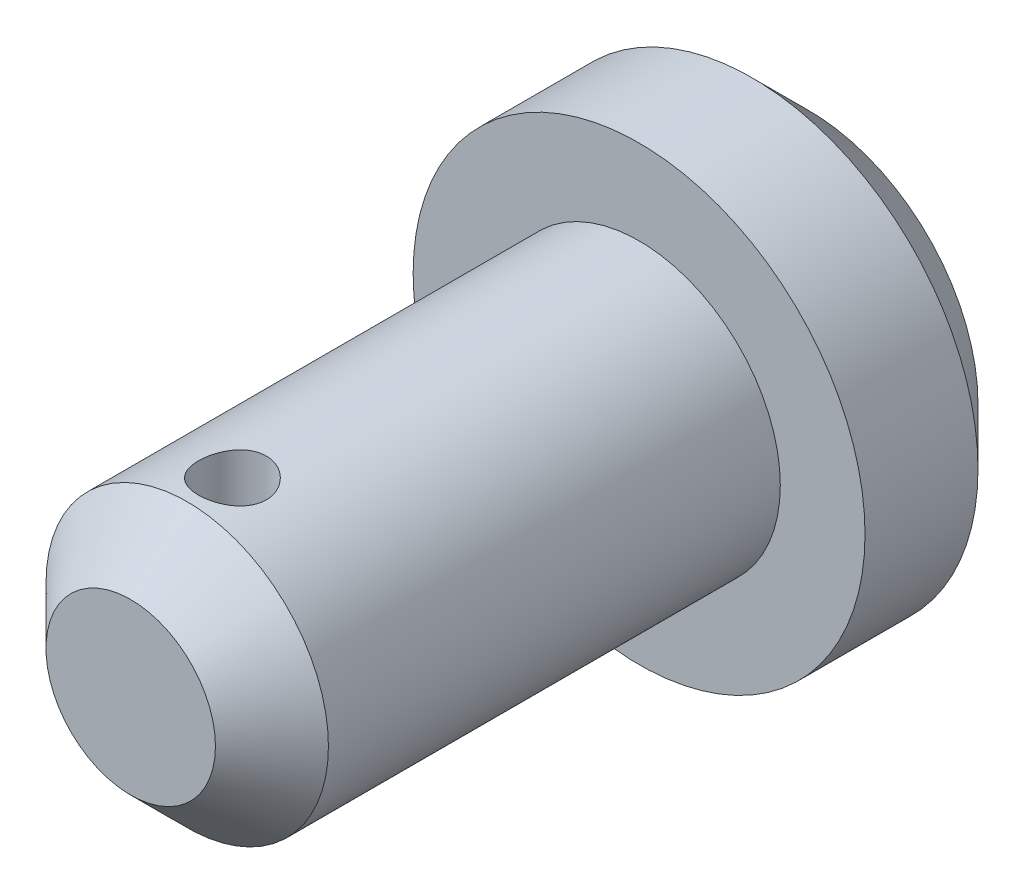
ISO-10303-21;
HEADER;
FILE_DESCRIPTION(('STEP AP214'),'2;1');
FILE_NAME('part.step','',(''),(''),'','','');
FILE_SCHEMA(('AUTOMOTIVE_DESIGN { 1 0 10303 214 1 1 1 1 }'));
ENDSEC;
DATA;
#1=APPLICATION_CONTEXT('core data for automotive mechanical design processes');
#2=APPLICATION_PROTOCOL_DEFINITION('international standard','automotive_design',2000,#1);
#3=PRODUCT_CONTEXT('',#1,'mechanical');
#4=PRODUCT('Part','Part','',(#3));
#5=PRODUCT_RELATED_PRODUCT_CATEGORY('part','',(#4));
#6=PRODUCT_DEFINITION_FORMATION('','',#4);
#7=PRODUCT_DEFINITION_CONTEXT('part definition',#1,'design');
#8=PRODUCT_DEFINITION('design','',#6,#7);
#9=PRODUCT_DEFINITION_SHAPE('','',#8);
#10=(LENGTH_UNIT() NAMED_UNIT(*) SI_UNIT(.MILLI.,.METRE.));
#11=(NAMED_UNIT(*) PLANE_ANGLE_UNIT() SI_UNIT($,.RADIAN.));
#12=(NAMED_UNIT(*) SI_UNIT($,.STERADIAN.) SOLID_ANGLE_UNIT());
#13=UNCERTAINTY_MEASURE_WITH_UNIT(LENGTH_MEASURE(1.E-05),#10,'distance_accuracy_value','');
#14=(GEOMETRIC_REPRESENTATION_CONTEXT(3) GLOBAL_UNCERTAINTY_ASSIGNED_CONTEXT((#13)) GLOBAL_UNIT_ASSIGNED_CONTEXT((#10,
#11,#12)) REPRESENTATION_CONTEXT('',''));
#15=CARTESIAN_POINT('',(0.,0.,0.));
#16=DIRECTION('',(0.,0.,1.));
#17=DIRECTION('',(1.,0.,0.));
#18=AXIS2_PLACEMENT_3D('',#15,#16,#17);
#19=CARTESIAN_POINT('',(0.,0.,30.));
#20=DIRECTION('',(0.,0.,-1.));
#21=DIRECTION('',(-1.,0.,0.));
#22=AXIS2_PLACEMENT_3D('',#19,#20,#21);
#23=CYLINDRICAL_SURFACE('',#22,40.);
#24=CARTESIAN_POINT('',(0.,0.,9.99999999999999));
#25=DIRECTION('',(0.,0.,1.));
#26=DIRECTION('',(1.,0.,0.));
#27=AXIS2_PLACEMENT_3D('',#24,#25,#26);
#28=CIRCLE('',#27,40.);
#29=CARTESIAN_POINT('',(40.,0.,9.99999999999999));
#30=VERTEX_POINT('',#29);
#31=EDGE_CURVE('E111',#30,#30,#28,.T.);
#32=ORIENTED_EDGE('',*,*,#31,.T.);
#33=EDGE_LOOP('',(#32));
#34=FACE_BOUND('',#33,.T.);
#35=CARTESIAN_POINT('',(0.,0.,30.));
#36=DIRECTION('',(0.,0.,1.));
#37=DIRECTION('',(1.,0.,0.));
#38=AXIS2_PLACEMENT_3D('',#35,#36,#37);
#39=CIRCLE('',#38,40.);
#40=CARTESIAN_POINT('',(40.,0.,30.));
#41=VERTEX_POINT('',#40);
#42=EDGE_CURVE('E115',#41,#41,#39,.T.);
#43=ORIENTED_EDGE('',*,*,#42,.F.);
#44=EDGE_LOOP('',(#43));
#45=FACE_BOUND('',#44,.T.);
#46=ADVANCED_FACE('F41',(#34,#45),#23,.T.);
#47=CARTESIAN_POINT('',(0.,0.,30.));
#48=DIRECTION('',(0.,0.,1.));
#49=DIRECTION('',(1.,0.,0.));
#50=AXIS2_PLACEMENT_3D('',#47,#48,#49);
#51=PLANE('',#50);
#52=CARTESIAN_POINT('',(0.,0.,30.));
#53=DIRECTION('',(0.,0.,1.));
#54=DIRECTION('',(1.,0.,0.));
#55=AXIS2_PLACEMENT_3D('',#52,#53,#54);
#56=CIRCLE('',#55,25.);
#57=CARTESIAN_POINT('',(25.,0.,30.));
#58=VERTEX_POINT('',#57);
#59=EDGE_CURVE('E120',#58,#58,#56,.F.);
#60=ORIENTED_EDGE('',*,*,#59,.T.);
#61=EDGE_LOOP('',(#60));
#62=FACE_BOUND('',#61,.T.);
#63=ORIENTED_EDGE('',*,*,#42,.T.);
#64=EDGE_LOOP('',(#63));
#65=FACE_BOUND('',#64,.T.);
#66=ADVANCED_FACE('F87',(#62,#65),#51,.T.);
#67=CARTESIAN_POINT('',(0.,0.,0.));
#68=DIRECTION('',(0.,0.,1.));
#69=DIRECTION('',(1.,0.,0.));
#70=AXIS2_PLACEMENT_3D('',#67,#68,#69);
#71=PLANE('',#70);
#72=CARTESIAN_POINT('',(0.,0.,0.));
#73=DIRECTION('',(0.,0.,1.));
#74=DIRECTION('',(1.,0.,0.));
#75=AXIS2_PLACEMENT_3D('',#72,#73,#74);
#76=CIRCLE('',#75,30.);
#77=CARTESIAN_POINT('',(30.,0.,0.));
#78=VERTEX_POINT('',#77);
#79=EDGE_CURVE('E58',#78,#78,#76,.F.);
#80=ORIENTED_EDGE('',*,*,#79,.T.);
#81=EDGE_LOOP('',(#80));
#82=FACE_BOUND('',#81,.T.);
#83=ADVANCED_FACE('F86',(#82),#71,.F.);
#84=CARTESIAN_POINT('',(0.,0.,120.));
#85=DIRECTION('',(0.,0.,-1.));
#86=DIRECTION('',(-1.,0.,0.));
#87=AXIS2_PLACEMENT_3D('',#84,#85,#86);
#88=CYLINDRICAL_SURFACE('',#87,25.);
#89=CARTESIAN_POINT('',(0.,-25.,108.));
#90=CARTESIAN_POINT('',(0.166017736340745,-25.0000026804997,108.000004565402));
#91=CARTESIAN_POINT('',(0.331984064130573,-24.9983437383731,107.99310833151));
#92=CARTESIAN_POINT('',(0.662757375273787,-24.9917601768854,107.965590990053));
#93=CARTESIAN_POINT('',(0.827564209779567,-24.9868351457074,107.944968151717));
#94=CARTESIAN_POINT('',(1.15483168687375,-24.9738504635424,107.890153584833));
#95=CARTESIAN_POINT('',(1.31729147606248,-24.9657897007271,107.855957043403));
#96=CARTESIAN_POINT('',(1.63872050759382,-24.9467537443302,107.77426192077));
#97=CARTESIAN_POINT('',(1.79768844089951,-24.9357774773038,107.726758439799));
#98=CARTESIAN_POINT('',(2.11072366381165,-24.9112316091515,107.618915400037));
#99=CARTESIAN_POINT('',(2.26479812859839,-24.897666030887,107.558595736763));
#100=CARTESIAN_POINT('',(2.56731972417304,-24.8682925860487,107.425512650401));
#101=CARTESIAN_POINT('',(2.71576475309531,-24.8524838922068,107.352744634275));
#102=CARTESIAN_POINT('',(3.00593509691774,-24.8190587739081,107.195342909448));
#103=CARTESIAN_POINT('',(3.14766294672407,-24.8014430394569,107.110713725361));
#104=CARTESIAN_POINT('',(3.42359889441686,-24.7648612187919,106.930128760191));
#105=CARTESIAN_POINT('',(3.55780414185137,-24.7458946268123,106.834168727859));
#106=CARTESIAN_POINT('',(3.81996752921304,-24.7067947855154,106.629894500437));
#107=CARTESIAN_POINT('',(3.94778319107672,-24.6866473068088,106.521400137686));
#108=CARTESIAN_POINT('',(4.19391043753481,-24.6460277155742,106.294087645878));
#109=CARTESIAN_POINT('',(4.31221847908385,-24.6255554853983,106.175265702235));
#110=CARTESIAN_POINT('',(4.53846894982134,-24.5848634527513,105.928149135848));
#111=CARTESIAN_POINT('',(4.64641408237688,-24.5646435856504,105.799856999123));
#112=CARTESIAN_POINT('',(4.85128465634762,-24.5250062264423,105.534563132888));
#113=CARTESIAN_POINT('',(4.94820601608993,-24.5055890332168,105.397558206456));
#114=CARTESIAN_POINT('',(5.1315149308875,-24.4678652790419,105.113910941245));
#115=CARTESIAN_POINT('',(5.21774615640803,-24.4495768107614,104.967165078552));
#116=CARTESIAN_POINT('',(5.37754406139993,-24.4149279468241,104.666645817285));
#117=CARTESIAN_POINT('',(5.45110595933349,-24.3985682798489,104.51286979304));
#118=CARTESIAN_POINT('',(5.58492026214268,-24.3682865029779,104.19946776603));
#119=CARTESIAN_POINT('',(5.64517912327472,-24.354363211339,104.039844645039));
#120=CARTESIAN_POINT('',(5.75195806967359,-24.3293636773731,103.715852874525));
#121=CARTESIAN_POINT('',(5.79847322039683,-24.318288457803,103.551482543759));
#122=CARTESIAN_POINT('',(5.91523377010968,-24.2902598679583,103.059199195839));
#123=CARTESIAN_POINT('',(5.96534620186163,-24.2778811042379,102.725874749114));
#124=CARTESIAN_POINT('',(5.99819895021149,-24.2697663322526,102.223524398244));
#125=CARTESIAN_POINT('',(6.00209048242324,-24.2688053008257,102.055614512631));
#126=CARTESIAN_POINT('',(5.99581246294927,-24.2703574949624,101.720053338741));
#127=CARTESIAN_POINT('',(5.98564275494965,-24.2728707591485,101.552402053359));
#128=CARTESIAN_POINT('',(5.93483975630033,-24.285368999466,101.059235437964));
#129=CARTESIAN_POINT('',(5.87440247397774,-24.3001939850224,100.73566109263));
#130=CARTESIAN_POINT('',(5.70184242669472,-24.3412549446464,100.103555140239));
#131=CARTESIAN_POINT('',(5.58971623816142,-24.3674916745551,99.7950245310886));
#132=CARTESIAN_POINT('',(5.31588253494411,-24.4286958367201,99.1981876883057));
#133=CARTESIAN_POINT('',(5.15371899452585,-24.4637429965247,98.9100987536133));
#134=CARTESIAN_POINT('',(4.78473374953622,-24.5385748778448,98.3647873385141));
#135=CARTESIAN_POINT('',(4.57790479882186,-24.5783603675971,98.1075698769834));
#136=CARTESIAN_POINT('',(4.11902988641842,-24.6594640880418,97.6242138778088));
#137=CARTESIAN_POINT('',(3.86594129003372,-24.7007951674045,97.3990660746998));
#138=CARTESIAN_POINT('',(3.32511184695823,-24.7793903091839,96.9942302876758));
#139=CARTESIAN_POINT('',(3.03737009894219,-24.8166542657671,96.8145434865743));
#140=CARTESIAN_POINT('',(2.43405695507431,-24.8830789940348,96.5054056318309));
#141=CARTESIAN_POINT('',(2.11840557448716,-24.9122154123614,96.3761051057317));
#142=CARTESIAN_POINT('',(1.46899521159138,-24.9589240940734,96.1726698236987));
#143=CARTESIAN_POINT('',(1.13523942521409,-24.9764983913503,96.0985253649671));
#144=CARTESIAN_POINT('',(0.467574800827578,-24.9978055089126,96.0089958704804));
#145=CARTESIAN_POINT('',(0.133856966575299,-25.0018564268946,95.9922601968733));
#146=CARTESIAN_POINT('',(-0.531608768658086,-24.9965614831509,96.0143335519038));
#147=CARTESIAN_POINT('',(-0.86335682994432,-24.9872167270307,96.053137996564));
#148=CARTESIAN_POINT('',(-1.51084514007902,-24.9563832816127,96.1840738854237));
#149=CARTESIAN_POINT('',(-1.82674108394961,-24.9350603275565,96.2754779523593));
#150=CARTESIAN_POINT('',(-2.43870667494971,-24.8826669936479,96.5081966502045));
#151=CARTESIAN_POINT('',(-2.73477441187556,-24.8515956762951,96.6495160816406));
#152=CARTESIAN_POINT('',(-3.30412273668565,-24.7823820658762,96.9807321749523));
#153=CARTESIAN_POINT('',(-3.57694246966835,-24.7441307708391,97.171397626969));
#154=CARTESIAN_POINT('',(-4.08719914724014,-24.6649871461435,97.5949176655097));
#155=CARTESIAN_POINT('',(-4.32463047973872,-24.6240943990594,97.8277789307352));
#156=CARTESIAN_POINT('',(-4.76284500809666,-24.5431489449983,98.3352671241417));
#157=CARTESIAN_POINT('',(-4.96268414096837,-24.5031358001301,98.6107154179113));
#158=CARTESIAN_POINT('',(-5.31333575577367,-24.4295058119813,99.1922356795911));
#159=CARTESIAN_POINT('',(-5.46415043292342,-24.395888682328,99.4983062754937));
#160=CARTESIAN_POINT('',(-5.64963439053452,-24.353347630646,99.9725936839859));
#161=CARTESIAN_POINT('',(-5.70458710242879,-24.3405033891164,100.132806956615));
#162=CARTESIAN_POINT('',(-5.80079732294279,-24.317755202926,100.457482020032));
#163=CARTESIAN_POINT('',(-5.84205998439172,-24.3078501521252,100.621942187143));
#164=CARTESIAN_POINT('',(-5.91053741786635,-24.2912903166139,100.953917903229));
#165=CARTESIAN_POINT('',(-5.93775173433046,-24.2846356373073,101.121433551105));
#166=CARTESIAN_POINT('',(-5.9778996520454,-24.2747841701866,101.458266466855));
#167=CARTESIAN_POINT('',(-5.99083389159896,-24.2715872278157,101.627583653861));
#168=CARTESIAN_POINT('',(-6.00215499594079,-24.2687899616173,101.962248730512));
#169=CARTESIAN_POINT('',(-6.00091722515412,-24.2690968340135,102.127583284474));
#170=CARTESIAN_POINT('',(-5.9848087278487,-24.2730742483489,102.457543521935));
#171=CARTESIAN_POINT('',(-5.96993829850501,-24.2767447169658,102.622169220808));
#172=CARTESIAN_POINT('',(-5.92668661056589,-24.2873399112073,102.949554601566));
#173=CARTESIAN_POINT('',(-5.89830323162515,-24.294265147542,103.112313986498));
#174=CARTESIAN_POINT('',(-5.82827196779405,-24.3111608262961,103.434730201481));
#175=CARTESIAN_POINT('',(-5.78662876790753,-24.3211301931022,103.59438810625));
#176=CARTESIAN_POINT('',(-5.69063662986336,-24.3437686465433,103.908807518971));
#177=CARTESIAN_POINT('',(-5.636348769168,-24.3564247302984,104.063588627183));
#178=CARTESIAN_POINT('',(-5.51539707483437,-24.3840980883562,104.367953388139));
#179=CARTESIAN_POINT('',(-5.44873755154826,-24.3991145400161,104.517538829599));
#180=CARTESIAN_POINT('',(-5.30348427217981,-24.4310987091682,104.810662166916));
#181=CARTESIAN_POINT('',(-5.22488523075194,-24.4480672900111,104.954197348336));
#182=CARTESIAN_POINT('',(-5.05635243091258,-24.4834782828489,105.234191145169));
#183=CARTESIAN_POINT('',(-4.96642242689348,-24.5019202059306,105.370652083515));
#184=CARTESIAN_POINT('',(-4.77346921711415,-24.5402505889388,105.638950383292));
#185=CARTESIAN_POINT('',(-4.67017903544833,-24.5601634300574,105.77059233113));
#186=CARTESIAN_POINT('',(-4.45304880482868,-24.600458146359,106.02470841849));
#187=CARTESIAN_POINT('',(-4.33921237965749,-24.6208398586377,106.147185681123));
#188=CARTESIAN_POINT('',(-4.10164015488732,-24.661530300392,106.382293112982));
#189=CARTESIAN_POINT('',(-3.97789855094998,-24.6818389796797,106.494917426377));
#190=CARTESIAN_POINT('',(-3.7214296777047,-24.7218081005976,106.709448104758));
#191=CARTESIAN_POINT('',(-3.58870570477299,-24.7414687761375,106.811358366933));
#192=CARTESIAN_POINT('',(-3.31280088827596,-24.7799327781137,107.005423922495));
#193=CARTESIAN_POINT('',(-3.16948213881108,-24.7987162302532,107.097387248362));
#194=CARTESIAN_POINT('',(-2.87543817634771,-24.8345280560803,107.268853072288));
#195=CARTESIAN_POINT('',(-2.72471571591035,-24.8515570748485,107.348360155973));
#196=CARTESIAN_POINT('',(-2.41692354679156,-24.883375777664,107.494312287148));
#197=CARTESIAN_POINT('',(-2.25985686316148,-24.8981665133663,107.560763473344));
#198=CARTESIAN_POINT('',(-1.94048744711081,-24.9250921884147,107.680104272039));
#199=CARTESIAN_POINT('',(-1.77818555787967,-24.9372275530119,107.732996056276));
#200=CARTESIAN_POINT('',(-1.35190448336007,-24.9647957983314,107.852025173454));
#201=CARTESIAN_POINT('',(-1.08469226075993,-24.9779181465939,107.907424148491));
#202=CARTESIAN_POINT('',(-0.5449403310719,-24.9955177731159,107.981406644206));
#203=CARTESIAN_POINT('',(-0.272400964328514,-24.9999956018512,107.999992509114));
#204=CARTESIAN_POINT('',(0.,-25.,108.));
#205=B_SPLINE_CURVE_WITH_KNOTS('',3,(#89,#90,#91,#92,#93,#94,#95,#96,#97,#98,#99,#100,#101,#102,
#103,#104,#105,#106,#107,#108,#109,#110,#111,#112,#113,#114,#115,#116,#117,#118,#119,#120,#121,
#122,#123,#124,#125,#126,#127,#128,#129,#130,#131,#132,#133,#134,#135,#136,#137,#138,#139,#140,
#141,#142,#143,#144,#145,#146,#147,#148,#149,#150,#151,#152,#153,#154,#155,#156,#157,#158,#159,
#160,#161,#162,#163,#164,#165,#166,#167,#168,#169,#170,#171,#172,#173,#174,#175,#176,#177,#178,
#179,#180,#181,#182,#183,#184,#185,#186,#187,#188,#189,#190,#191,#192,#193,#194,#195,#196,#197,
#198,#199,#200,#201,#202,#203,#204),.UNSPECIFIED.,.T.,.F.,(4,2,2,2,2,2,2,2,2,2,2,2,2,2,2,2,2,2,
2,2,2,2,2,2,2,2,2,2,2,2,2,2,2,2,2,2,2,2,2,2,2,2,2,2,2,2,2,2,2,2,2,2,2,2,2,2,2,4),(0.,
0.497813360100957,0.995689500769752,1.49374233325073,1.9919787960947,2.4894473877073,
2.98709992652941,3.48456314269131,3.98221359994715,4.48820831908743,4.99439073274953,
5.50044073797178,6.00667750796929,6.51961190143619,7.03273945954077,7.54561743540081,
8.05867933189508,9.06463756237655,9.56800871792684,10.0713854693234,11.0548629550303,
12.0384055899336,13.0311908061742,14.0241372047509,15.0430966233895,16.0620825507942,
17.0840897493149,18.1059171185591,19.1035329919673,20.1010665323702,21.085126203147,
22.069280539993,23.0698021185097,24.0704821968969,25.0936623603892,26.1167967016263,
26.6258643414059,27.1347401541085,27.6436324676663,28.1525020334114,28.6479253897996,
29.1433379468293,29.6388282657176,30.1341437102249,30.6271145113295,31.1199138801487,
31.6129320389054,32.105787268885,32.6107272666004,33.1154944014541,33.6205595212516,
34.1254402854413,34.6387770201077,35.1519243293048,35.6648297831432,36.177653036205,
36.9945144051894,37.8113237554193),.UNSPECIFIED.);
#206=CARTESIAN_POINT('',(0.,-25.,108.));
#207=VERTEX_POINT('',#206);
#208=EDGE_CURVE('E46',#207,#207,#205,.T.);
#209=ORIENTED_EDGE('',*,*,#208,.T.);
#210=EDGE_LOOP('',(#209));
#211=FACE_BOUND('',#210,.T.);
#212=CARTESIAN_POINT('',(0.,25.,108.));
#213=CARTESIAN_POINT('',(-0.166017736340745,25.0000026804997,108.000004565402));
#214=CARTESIAN_POINT('',(-0.331984064130573,24.9983437383731,107.99310833151));
#215=CARTESIAN_POINT('',(-0.662757375273787,24.9917601768854,107.965590990053));
#216=CARTESIAN_POINT('',(-0.827564209779567,24.9868351457074,107.944968151717));
#217=CARTESIAN_POINT('',(-1.15483168687375,24.9738504635424,107.890153584833));
#218=CARTESIAN_POINT('',(-1.31729147606248,24.9657897007271,107.855957043403));
#219=CARTESIAN_POINT('',(-1.63872050759382,24.9467537443302,107.77426192077));
#220=CARTESIAN_POINT('',(-1.79768844089951,24.9357774773038,107.726758439799));
#221=CARTESIAN_POINT('',(-2.11072366381165,24.9112316091515,107.618915400037));
#222=CARTESIAN_POINT('',(-2.26479812859839,24.897666030887,107.558595736763));
#223=CARTESIAN_POINT('',(-2.56731972417305,24.8682925860487,107.425512650401));
#224=CARTESIAN_POINT('',(-2.71576475309531,24.8524838922068,107.352744634275));
#225=CARTESIAN_POINT('',(-3.00593509691775,24.8190587739081,107.195342909448));
#226=CARTESIAN_POINT('',(-3.14766294672408,24.8014430394569,107.110713725361));
#227=CARTESIAN_POINT('',(-3.42359889441686,24.7648612187919,106.930128760191));
#228=CARTESIAN_POINT('',(-3.55780414185137,24.7458946268123,106.834168727859));
#229=CARTESIAN_POINT('',(-3.81996752921304,24.7067947855154,106.629894500437));
#230=CARTESIAN_POINT('',(-3.94778319107672,24.6866473068088,106.521400137686));
#231=CARTESIAN_POINT('',(-4.19391043753481,24.6460277155742,106.294087645878));
#232=CARTESIAN_POINT('',(-4.31221847908385,24.6255554853983,106.175265702235));
#233=CARTESIAN_POINT('',(-4.53846894982134,24.5848634527513,105.928149135848));
#234=CARTESIAN_POINT('',(-4.64641408237688,24.5646435856504,105.799856999123));
#235=CARTESIAN_POINT('',(-4.85128465634762,24.5250062264423,105.534563132888));
#236=CARTESIAN_POINT('',(-4.94820601608993,24.5055890332168,105.397558206456));
#237=CARTESIAN_POINT('',(-5.1315149308875,24.4678652790419,105.113910941245));
#238=CARTESIAN_POINT('',(-5.21774615640803,24.4495768107614,104.967165078552));
#239=CARTESIAN_POINT('',(-5.37754406139993,24.4149279468241,104.666645817285));
#240=CARTESIAN_POINT('',(-5.45110595933349,24.3985682798489,104.51286979304));
#241=CARTESIAN_POINT('',(-5.58492026214268,24.3682865029779,104.19946776603));
#242=CARTESIAN_POINT('',(-5.64517912327472,24.354363211339,104.039844645039));
#243=CARTESIAN_POINT('',(-5.75195806967359,24.3293636773731,103.715852874525));
#244=CARTESIAN_POINT('',(-5.79847322039683,24.318288457803,103.551482543759));
#245=CARTESIAN_POINT('',(-5.91523377010968,24.2902598679583,103.059199195839));
#246=CARTESIAN_POINT('',(-5.96534620186163,24.2778811042379,102.725874749114));
#247=CARTESIAN_POINT('',(-5.99819895021149,24.2697663322526,102.223524398244));
#248=CARTESIAN_POINT('',(-6.00209048242324,24.2688053008257,102.055614512631));
#249=CARTESIAN_POINT('',(-5.99581246294927,24.2703574949624,101.720053338741));
#250=CARTESIAN_POINT('',(-5.98564275494965,24.2728707591485,101.552402053359));
#251=CARTESIAN_POINT('',(-5.93483975630033,24.285368999466,101.059235437964));
#252=CARTESIAN_POINT('',(-5.87440247397774,24.3001939850224,100.73566109263));
#253=CARTESIAN_POINT('',(-5.70184242669472,24.3412549446464,100.103555140239));
#254=CARTESIAN_POINT('',(-5.58971623816142,24.3674916745551,99.7950245310886));
#255=CARTESIAN_POINT('',(-5.31588253494411,24.4286958367201,99.1981876883057));
#256=CARTESIAN_POINT('',(-5.15371899452585,24.4637429965247,98.9100987536133));
#257=CARTESIAN_POINT('',(-4.78473374953622,24.5385748778448,98.3647873385141));
#258=CARTESIAN_POINT('',(-4.57790479882186,24.5783603675971,98.1075698769834));
#259=CARTESIAN_POINT('',(-4.11902988641842,24.6594640880418,97.6242138778088));
#260=CARTESIAN_POINT('',(-3.86594129003372,24.7007951674045,97.3990660746998));
#261=CARTESIAN_POINT('',(-3.32511184695823,24.7793903091839,96.9942302876758));
#262=CARTESIAN_POINT('',(-3.03737009894219,24.8166542657671,96.8145434865743));
#263=CARTESIAN_POINT('',(-2.43405695507431,24.8830789940348,96.5054056318309));
#264=CARTESIAN_POINT('',(-2.11840557448716,24.9122154123614,96.3761051057317));
#265=CARTESIAN_POINT('',(-1.46899521159138,24.9589240940734,96.1726698236987));
#266=CARTESIAN_POINT('',(-1.13523942521409,24.9764983913503,96.0985253649671));
#267=CARTESIAN_POINT('',(-0.467574800827579,24.9978055089126,96.0089958704804));
#268=CARTESIAN_POINT('',(-0.133856966575301,25.0018564268946,95.9922601968733));
#269=CARTESIAN_POINT('',(0.531608768658084,24.9965614831509,96.0143335519038));
#270=CARTESIAN_POINT('',(0.863356829944318,24.9872167270307,96.053137996564));
#271=CARTESIAN_POINT('',(1.51084514007902,24.9563832816127,96.1840738854237));
#272=CARTESIAN_POINT('',(1.82674108394961,24.9350603275565,96.2754779523593));
#273=CARTESIAN_POINT('',(2.43870667494971,24.8826669936479,96.5081966502045));
#274=CARTESIAN_POINT('',(2.73477441187556,24.8515956762951,96.6495160816406));
#275=CARTESIAN_POINT('',(3.30412273668565,24.7823820658762,96.9807321749523));
#276=CARTESIAN_POINT('',(3.57694246966835,24.7441307708391,97.171397626969));
#277=CARTESIAN_POINT('',(4.08719914724014,24.6649871461435,97.5949176655097));
#278=CARTESIAN_POINT('',(4.32463047973873,24.6240943990594,97.8277789307352));
#279=CARTESIAN_POINT('',(4.76284500809667,24.5431489449983,98.3352671241417));
#280=CARTESIAN_POINT('',(4.96268414096837,24.5031358001301,98.6107154179113));
#281=CARTESIAN_POINT('',(5.31333575577368,24.4295058119813,99.1922356795911));
#282=CARTESIAN_POINT('',(5.46415043292342,24.395888682328,99.4983062754937));
#283=CARTESIAN_POINT('',(5.64963439053452,24.353347630646,99.9725936839859));
#284=CARTESIAN_POINT('',(5.70458710242879,24.3405033891164,100.132806956615));
#285=CARTESIAN_POINT('',(5.80079732294279,24.317755202926,100.457482020032));
#286=CARTESIAN_POINT('',(5.84205998439172,24.3078501521252,100.621942187143));
#287=CARTESIAN_POINT('',(5.91053741786635,24.2912903166139,100.953917903229));
#288=CARTESIAN_POINT('',(5.93775173433046,24.2846356373073,101.121433551105));
#289=CARTESIAN_POINT('',(5.9778996520454,24.2747841701866,101.458266466855));
#290=CARTESIAN_POINT('',(5.99083389159896,24.2715872278157,101.627583653861));
#291=CARTESIAN_POINT('',(6.00215499594079,24.2687899616173,101.962248730512));
#292=CARTESIAN_POINT('',(6.00091722515412,24.2690968340135,102.127583284474));
#293=CARTESIAN_POINT('',(5.9848087278487,24.2730742483489,102.457543521935));
#294=CARTESIAN_POINT('',(5.96993829850501,24.2767447169658,102.622169220808));
#295=CARTESIAN_POINT('',(5.92668661056589,24.2873399112073,102.949554601566));
#296=CARTESIAN_POINT('',(5.89830323162515,24.294265147542,103.112313986498));
#297=CARTESIAN_POINT('',(5.82827196779405,24.3111608262961,103.434730201481));
#298=CARTESIAN_POINT('',(5.78662876790753,24.3211301931022,103.59438810625));
#299=CARTESIAN_POINT('',(5.69063662986336,24.3437686465433,103.908807518971));
#300=CARTESIAN_POINT('',(5.636348769168,24.3564247302984,104.063588627183));
#301=CARTESIAN_POINT('',(5.51539707483437,24.3840980883562,104.367953388139));
#302=CARTESIAN_POINT('',(5.44873755154826,24.3991145400161,104.517538829599));
#303=CARTESIAN_POINT('',(5.30348427217981,24.4310987091682,104.810662166916));
#304=CARTESIAN_POINT('',(5.22488523075194,24.4480672900111,104.954197348336));
#305=CARTESIAN_POINT('',(5.05635243091257,24.4834782828489,105.234191145169));
#306=CARTESIAN_POINT('',(4.96642242689347,24.5019202059306,105.370652083515));
#307=CARTESIAN_POINT('',(4.77346921711415,24.5402505889388,105.638950383292));
#308=CARTESIAN_POINT('',(4.67017903544834,24.5601634300573,105.77059233113));
#309=CARTESIAN_POINT('',(4.45304880482869,24.600458146359,106.02470841849));
#310=CARTESIAN_POINT('',(4.33921237965749,24.6208398586377,106.147185681123));
#311=CARTESIAN_POINT('',(4.10164015488731,24.661530300392,106.382293112982));
#312=CARTESIAN_POINT('',(3.97789855094998,24.6818389796797,106.494917426377));
#313=CARTESIAN_POINT('',(3.7214296777047,24.7218081005976,106.709448104758));
#314=CARTESIAN_POINT('',(3.58870570477299,24.7414687761375,106.811358366933));
#315=CARTESIAN_POINT('',(3.31280088827595,24.7799327781137,107.005423922495));
#316=CARTESIAN_POINT('',(3.16948213881108,24.7987162302532,107.097387248362));
#317=CARTESIAN_POINT('',(2.8754381763477,24.8345280560803,107.268853072288));
#318=CARTESIAN_POINT('',(2.72471571591034,24.8515570748485,107.348360155973));
#319=CARTESIAN_POINT('',(2.41692354679156,24.883375777664,107.494312287148));
#320=CARTESIAN_POINT('',(2.25985686316148,24.8981665133663,107.560763473344));
#321=CARTESIAN_POINT('',(1.94048744711082,24.9250921884147,107.680104272039));
#322=CARTESIAN_POINT('',(1.77818555787967,24.9372275530119,107.732996056276));
#323=CARTESIAN_POINT('',(1.35190448336007,24.9647957983314,107.852025173454));
#324=CARTESIAN_POINT('',(1.08469226075993,24.9779181465939,107.907424148491));
#325=CARTESIAN_POINT('',(0.544940331071899,24.9955177731159,107.981406644206));
#326=CARTESIAN_POINT('',(0.272400964328514,24.9999956018512,107.999992509114));
#327=CARTESIAN_POINT('',(0.,25.,108.));
#328=B_SPLINE_CURVE_WITH_KNOTS('',3,(#212,#213,#214,#215,#216,#217,#218,#219,#220,#221,#222,
#223,#224,#225,#226,#227,#228,#229,#230,#231,#232,#233,#234,#235,#236,#237,#238,#239,#240,#241,
#242,#243,#244,#245,#246,#247,#248,#249,#250,#251,#252,#253,#254,#255,#256,#257,#258,#259,#260,
#261,#262,#263,#264,#265,#266,#267,#268,#269,#270,#271,#272,#273,#274,#275,#276,#277,#278,#279,
#280,#281,#282,#283,#284,#285,#286,#287,#288,#289,#290,#291,#292,#293,#294,#295,#296,#297,#298,
#299,#300,#301,#302,#303,#304,#305,#306,#307,#308,#309,#310,#311,#312,#313,#314,#315,#316,#317,
#318,#319,#320,#321,#322,#323,#324,#325,#326,#327),.UNSPECIFIED.,.T.,.F.,(4,2,2,2,2,2,2,2,2,2,2,
2,2,2,2,2,2,2,2,2,2,2,2,2,2,2,2,2,2,2,2,2,2,2,2,2,2,2,2,2,2,2,2,2,2,2,2,2,2,2,2,2,2,2,2,2,2,4),
(0.,0.497813360100957,0.995689500769752,1.49374233325073,1.9919787960947,2.4894473877073,
2.98709992652941,3.48456314269131,3.98221359994715,4.48820831908743,4.99439073274953,
5.50044073797178,6.00667750796929,6.51961190143619,7.03273945954077,7.54561743540081,
8.05867933189508,9.06463756237655,9.56800871792684,10.0713854693234,11.0548629550303,
12.0384055899336,13.0311908061742,14.0241372047509,15.0430966233895,16.0620825507942,
17.0840897493149,18.1059171185591,19.1035329919673,20.1010665323702,21.085126203147,
22.069280539993,23.0698021185097,24.0704821968969,25.0936623603893,26.1167967016263,
26.6258643414059,27.1347401541085,27.6436324676663,28.1525020334114,28.6479253897996,
29.1433379468293,29.6388282657176,30.1341437102249,30.6271145113295,31.1199138801487,
31.6129320389054,32.105787268885,32.6107272666004,33.1154944014541,33.6205595212516,
34.1254402854413,34.6387770201077,35.1519243293048,35.6648297831432,36.177653036205,
36.9945144051894,37.8113237554193),.UNSPECIFIED.);
#329=CARTESIAN_POINT('',(0.,25.,108.));
#330=VERTEX_POINT('',#329);
#331=EDGE_CURVE('E64',#330,#330,#328,.T.);
#332=ORIENTED_EDGE('',*,*,#331,.T.);
#333=EDGE_LOOP('',(#332));
#334=FACE_BOUND('',#333,.T.);
#335=CARTESIAN_POINT('',(0.,0.,110.));
#336=DIRECTION('',(0.,0.,1.));
#337=DIRECTION('',(1.,0.,0.));
#338=AXIS2_PLACEMENT_3D('',#335,#336,#337);
#339=CIRCLE('',#338,25.);
#340=CARTESIAN_POINT('',(25.,0.,110.));
#341=VERTEX_POINT('',#340);
#342=EDGE_CURVE('E10',#341,#341,#339,.F.);
#343=ORIENTED_EDGE('',*,*,#342,.T.);
#344=EDGE_LOOP('',(#343));
#345=FACE_BOUND('',#344,.T.);
#346=ORIENTED_EDGE('',*,*,#59,.F.);
#347=EDGE_LOOP('',(#346));
#348=FACE_BOUND('',#347,.T.);
#349=ADVANCED_FACE('F70',(#211,#334,#345,#348),#88,.T.);
#350=CARTESIAN_POINT('',(0.,0.,120.));
#351=DIRECTION('',(0.,0.,1.));
#352=DIRECTION('',(1.,0.,0.));
#353=AXIS2_PLACEMENT_3D('',#350,#351,#352);
#354=PLANE('',#353);
#355=CARTESIAN_POINT('',(0.,0.,120.));
#356=DIRECTION('',(0.,0.,1.));
#357=DIRECTION('',(1.,0.,0.));
#358=AXIS2_PLACEMENT_3D('',#355,#356,#357);
#359=CIRCLE('',#358,15.0000000000001);
#360=CARTESIAN_POINT('',(15.0000000000001,0.,120.));
#361=VERTEX_POINT('',#360);
#362=EDGE_CURVE('E54',#361,#361,#359,.T.);
#363=ORIENTED_EDGE('',*,*,#362,.T.);
#364=EDGE_LOOP('',(#363));
#365=FACE_BOUND('',#364,.T.);
#366=ADVANCED_FACE('F77',(#365),#354,.T.);
#367=CARTESIAN_POINT('',(0.,0.,9.99999999999999));
#368=DIRECTION('',(0.,0.,1.));
#369=DIRECTION('',(1.,0.,0.));
#370=AXIS2_PLACEMENT_3D('',#367,#368,#369);
#371=CONICAL_SURFACE('',#370,40.,0.78539816339745);
#372=CARTESIAN_POINT('',(30.,0.,0.));
#373=CARTESIAN_POINT('',(30.1041666666666,0.,0.104166666666665));
#374=CARTESIAN_POINT('',(30.2083333333333,0.,0.208333333333332));
#375=CARTESIAN_POINT('',(30.4166666666666,0.,0.416666666666665));
#376=CARTESIAN_POINT('',(30.5208333333333,0.,0.520833333333331));
#377=CARTESIAN_POINT('',(30.7291666666666,0.,0.729166666666664));
#378=CARTESIAN_POINT('',(30.8333333333333,0.,0.83333333333333));
#379=CARTESIAN_POINT('',(31.0416666666666,0.,1.04166666666666));
#380=CARTESIAN_POINT('',(31.1458333333333,0.,1.14583333333333));
#381=CARTESIAN_POINT('',(31.3541666666666,0.,1.35416666666666));
#382=CARTESIAN_POINT('',(31.4583333333333,0.,1.45833333333333));
#383=CARTESIAN_POINT('',(31.6666666666666,0.,1.66666666666666));
#384=CARTESIAN_POINT('',(31.7708333333333,0.,1.77083333333333));
#385=CARTESIAN_POINT('',(31.9791666666666,0.,1.97916666666666));
#386=CARTESIAN_POINT('',(32.0833333333333,0.,2.08333333333333));
#387=CARTESIAN_POINT('',(32.2916666666666,0.,2.29166666666666));
#388=CARTESIAN_POINT('',(32.3958333333333,0.,2.39583333333333));
#389=CARTESIAN_POINT('',(32.6041666666666,0.,2.60416666666666));
#390=CARTESIAN_POINT('',(32.7083333333333,0.,2.70833333333333));
#391=CARTESIAN_POINT('',(32.9166666666666,0.,2.91666666666666));
#392=CARTESIAN_POINT('',(33.0208333333333,0.,3.02083333333333));
#393=CARTESIAN_POINT('',(33.2291666666667,0.,3.22916666666666));
#394=CARTESIAN_POINT('',(33.3333333333333,0.,3.33333333333333));
#395=CARTESIAN_POINT('',(33.5416666666667,0.,3.54166666666666));
#396=CARTESIAN_POINT('',(33.6458333333333,0.,3.64583333333333));
#397=CARTESIAN_POINT('',(33.8541666666667,0.,3.85416666666666));
#398=CARTESIAN_POINT('',(33.9583333333333,0.,3.95833333333333));
#399=CARTESIAN_POINT('',(34.1666666666667,0.,4.16666666666666));
#400=CARTESIAN_POINT('',(34.2708333333333,0.,4.27083333333333));
#401=CARTESIAN_POINT('',(34.4791666666667,0.,4.47916666666666));
#402=CARTESIAN_POINT('',(34.5833333333333,0.,4.58333333333333));
#403=CARTESIAN_POINT('',(34.7916666666667,0.,4.79166666666666));
#404=CARTESIAN_POINT('',(34.8958333333333,0.,4.89583333333333));
#405=CARTESIAN_POINT('',(35.1041666666667,0.,5.10416666666666));
#406=CARTESIAN_POINT('',(35.2083333333333,0.,5.20833333333333));
#407=CARTESIAN_POINT('',(35.4166666666667,0.,5.41666666666666));
#408=CARTESIAN_POINT('',(35.5208333333333,0.,5.52083333333333));
#409=CARTESIAN_POINT('',(35.7291666666667,0.,5.72916666666666));
#410=CARTESIAN_POINT('',(35.8333333333333,0.,5.83333333333333));
#411=CARTESIAN_POINT('',(36.0416666666667,0.,6.04166666666666));
#412=CARTESIAN_POINT('',(36.1458333333333,0.,6.14583333333333));
#413=CARTESIAN_POINT('',(36.3541666666667,0.,6.35416666666666));
#414=CARTESIAN_POINT('',(36.4583333333333,0.,6.45833333333333));
#415=CARTESIAN_POINT('',(36.6666666666667,0.,6.66666666666666));
#416=CARTESIAN_POINT('',(36.7708333333333,0.,6.77083333333332));
#417=CARTESIAN_POINT('',(36.9791666666667,0.,6.97916666666666));
#418=CARTESIAN_POINT('',(37.0833333333333,0.,7.08333333333332));
#419=CARTESIAN_POINT('',(37.2916666666667,0.,7.29166666666666));
#420=CARTESIAN_POINT('',(37.3958333333333,0.,7.39583333333332));
#421=CARTESIAN_POINT('',(37.6041666666667,0.,7.60416666666666));
#422=CARTESIAN_POINT('',(37.7083333333333,0.,7.70833333333332));
#423=CARTESIAN_POINT('',(37.9166666666667,0.,7.91666666666666));
#424=CARTESIAN_POINT('',(38.0208333333333,0.,8.02083333333333));
#425=CARTESIAN_POINT('',(38.2291666666667,0.,8.22916666666666));
#426=CARTESIAN_POINT('',(38.3333333333333,0.,8.33333333333332));
#427=CARTESIAN_POINT('',(38.5416666666667,0.,8.54166666666666));
#428=CARTESIAN_POINT('',(38.6458333333333,0.,8.64583333333332));
#429=CARTESIAN_POINT('',(38.8541666666667,0.,8.85416666666666));
#430=CARTESIAN_POINT('',(38.9583333333333,0.,8.95833333333332));
#431=CARTESIAN_POINT('',(39.1666666666667,0.,9.16666666666666));
#432=CARTESIAN_POINT('',(39.2708333333333,0.,9.27083333333332));
#433=CARTESIAN_POINT('',(39.4791666666667,0.,9.47916666666666));
#434=CARTESIAN_POINT('',(39.5833333333333,0.,9.58333333333332));
#435=CARTESIAN_POINT('',(39.7916666666667,0.,9.79166666666665));
#436=CARTESIAN_POINT('',(39.8958333333333,0.,9.89583333333332));
#437=CARTESIAN_POINT('',(40.,0.,9.99999999999999));
#438=B_SPLINE_CURVE_WITH_KNOTS('',3,(#372,#373,#374,#375,#376,#377,#378,#379,#380,#381,#382,
#383,#384,#385,#386,#387,#388,#389,#390,#391,#392,#393,#394,#395,#396,#397,#398,#399,#400,#401,
#402,#403,#404,#405,#406,#407,#408,#409,#410,#411,#412,#413,#414,#415,#416,#417,#418,#419,#420,
#421,#422,#423,#424,#425,#426,#427,#428,#429,#430,#431,#432,#433,#434,#435,#436,#437),
.UNSPECIFIED.,.F.,.F.,(4,2,2,2,2,2,2,2,2,2,2,2,2,2,2,2,2,2,2,2,2,2,2,2,2,2,2,2,2,2,2,2,4),(0.,
0.441941738241593,0.883883476483184,1.32582521472478,1.76776695296637,2.20970869120796,
2.65165042944956,3.09359216769115,3.53553390593274,3.97747564417433,4.41941738241593,
4.86135912065752,5.30330085889911,5.74524259714071,6.1871843353823,6.62912607362389,
7.07106781186548,7.51300955010708,7.95495128834867,8.39689302659026,8.83883476483186,
9.28077650307345,9.72271824131504,10.1646599795566,10.6066017177982,11.0485434560398,
11.4904851942814,11.932426932523,12.3743686707646,12.8163104090062,13.2582521472478,
13.7001938854894,14.142135623731),.UNSPECIFIED.);
#439=EDGE_CURVE('BSEAM79',#78,#30,#438,.T.);
#440=ORIENTED_EDGE('',*,*,#79,.F.);
#441=ORIENTED_EDGE('',*,*,#31,.F.);
#442=ORIENTED_EDGE('',*,*,#439,.T.);
#443=ORIENTED_EDGE('',*,*,#439,.F.);
#444=EDGE_LOOP('',(#440,#442,#441,#443));
#445=FACE_BOUND('',#444,.T.);
#446=ADVANCED_FACE('F79',(#445),#371,.T.);
#447=CARTESIAN_POINT('',(0.,0.,120.));
#448=DIRECTION('',(0.,0.,-1.));
#449=DIRECTION('',(-1.,0.,0.));
#450=AXIS2_PLACEMENT_3D('',#447,#448,#449);
#451=CONICAL_SURFACE('',#450,15.0000000000001,0.785398163397448);
#452=ORIENTED_EDGE('',*,*,#342,.F.);
#453=EDGE_LOOP('',(#452));
#454=FACE_BOUND('',#453,.T.);
#455=ORIENTED_EDGE('',*,*,#362,.F.);
#456=EDGE_LOOP('',(#455));
#457=FACE_BOUND('',#456,.T.);
#458=ADVANCED_FACE('F42',(#454,#457),#451,.T.);
#459=CARTESIAN_POINT('',(0.,-30.,102.));
#460=DIRECTION('',(0.,1.,0.));
#461=DIRECTION('',(0.,0.,1.));
#462=AXIS2_PLACEMENT_3D('',#459,#460,#461);
#463=CYLINDRICAL_SURFACE('',#462,6.00000000000001);
#464=ORIENTED_EDGE('',*,*,#331,.F.);
#465=EDGE_LOOP('',(#464));
#466=FACE_BOUND('',#465,.T.);
#467=ORIENTED_EDGE('',*,*,#208,.F.);
#468=EDGE_LOOP('',(#467));
#469=FACE_BOUND('',#468,.T.);
#470=ADVANCED_FACE('F75',(#466,#469),#463,.F.);
#471=CLOSED_SHELL('',(#46,#66,#83,#349,#366,#446,#458,#470));
#472=MANIFOLD_SOLID_BREP('B2',#471);
#473=ADVANCED_BREP_SHAPE_REPRESENTATION('',(#18,#472),#14);
#474=SHAPE_DEFINITION_REPRESENTATION(#9,#473);
ENDSEC;
END-ISO-10303-21;
